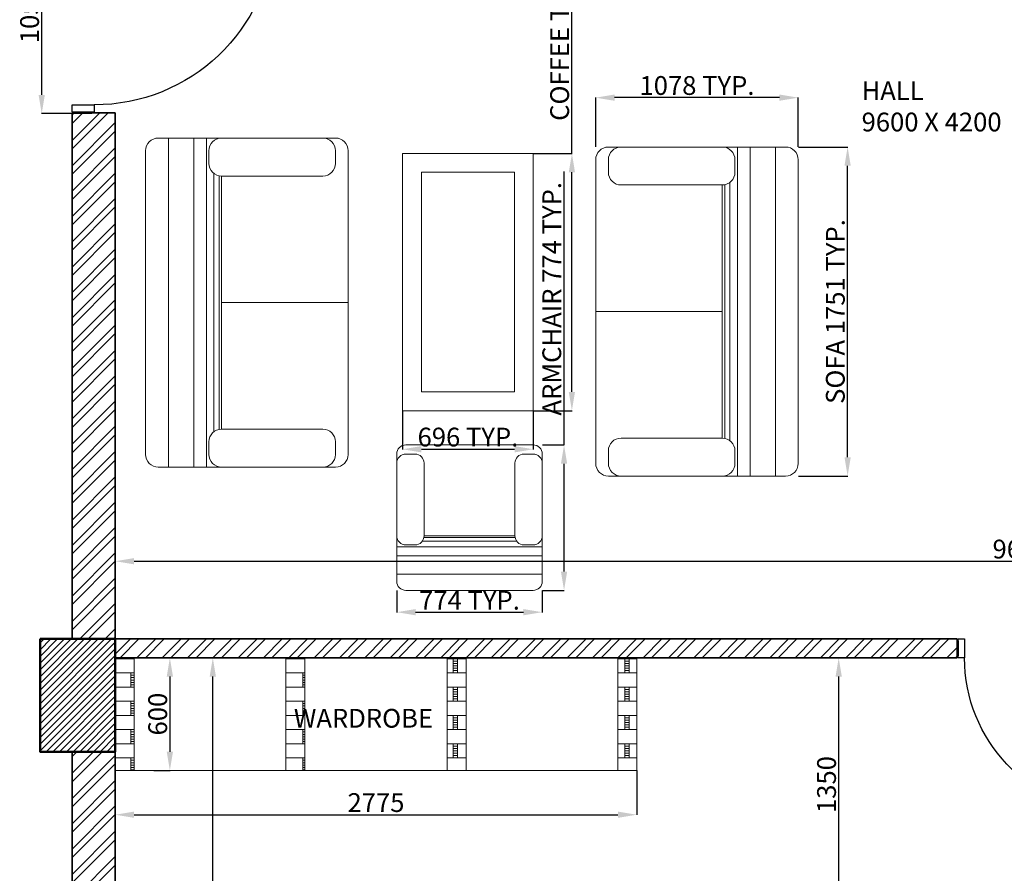
# Model space of a CAD drawing. Units: millimetres. Extents: x -3326 to 29338, y -16792 to 6002.
# Tile 17 of 21: x 17004 to 22244, y -7931 to -3388. Entities that reach past the tile are written whole.
import ezdxf

# ---------------------------------------------------------------- set-up
doc = ezdxf.new("R2010")
doc.units = ezdxf.units.MM
doc.header["$PDMODE"] = 35
doc.header["$PDSIZE"] = 5
for name, color, linetype, lineweight in [('A-ANNO-DIMS', 2, 'Continuous', 13), ('A-AREA-IDEN', 7, 'Continuous', 18), ('A-COLS', 1, 'Continuous', 50), ('A-COLS-PATT', 251, 'Continuous', 13), ('A-DOOR', 3, 'Continuous', 25), ('A-FLOR-CASE', 30, 'Continuous', 18), ('A-FLOR-CASE-PATT', 252, 'Continuous', 13), ('A-WALL', 7, 'Continuous', 35), ('A-WALL-PATT', 252, 'Continuous', 13), ('furn', 28, 'Continuous', 18), ('txt', 7, 'Continuous', 18)]:
    doc.layers.add(name, color=color, linetype=linetype, lineweight=lineweight)
doc.styles.get("Standard").update_dxf_attribs({"font": 'arial.ttf'})
doc.dimstyles.new('ISO-25', dxfattribs={"dimtxt": 100, "dimasz": 100, "dimexe": 1.25, "dimexo": 0.625, "dimtad": 1, "dimtxsty": 'Standard', "dimcen": 2.5, "dimadec": 0, "dimazin": 0, "dimtfac": 1, "dimtmove": 0, "dimatfit": 3, "dimfxl": 1, "dimarcsym": 0})

# ---------------------------------------------------------------- blocks, each defined once
blk = doc.blocks.new('A$C0CE462CD')
for p, q in [((860, 100), (860, 0)), ((860, 0), (893.9, 0))]:
    blk.add_line(p, q)
for points in [[(860, 100), (860, 920), (818.4, 920), (818.4, 100)], [(0, 10), (6.1, 10), (6.1, 90), (0, 90)], [(893.9, 10), (900, 10), (900, 90), (893.9, 90)]]:
    blk.add_lwpolyline(points, close=True)
for points in [[(6.1, 0), (40, 0), (40, 100), (6.1, 100)], [(6.1, 100), (6.1, 0)], [(860, 100), (893.9, 100), (893.9, 0)]]:
    blk.add_lwpolyline(points)
blk.add_arc((859.1, 101.9), 819.1, 92.8508, 180.1309)
blk = doc.blocks.new('sofa-29')
at = {"color": 0, "linetype": 'ByBlock'}
for p, q in [((1.2, 0.8), (0, 0.8)), ((0.6, 0.8), (0.6, 0.3)), ((-0.05, 0.05), (-0.05, 0.75)), ((-0.05, 0.05), (-0.05, 0.75)), ((0, 0.75), (0.05, 0.75)), ((1.2, 0.75), (1.15, 0.75)), ((1.25, 0.05), (1.25, 0.75)), ((0.1, 0.3), (0.1, 0.7)), ((1.1, 0.3), (1.1, 0.7)), ((1.1, 0.29), (0.099, 0.29)), ((1.1, 0.3), (0.1, 0.3)), ((1.25, 0.24), (-0.05, 0.24)), ((0, 0.25), (0.05, 0.25)), ((1.11, 0.27), (0.09, 0.27)), ((1.2, 0.25), (1.15, 0.25)), ((1.25, 0.19), (-0.05, 0.19)), ((1.25, 0.09), (-0.05, 0.09)), ((1.2, 0), (0, 0))]:
    blk.add_line(p, q, dxfattribs=at)
for centre, start, end in [((0, 0.75), 90, 180), ((1.2, 0.75), 0, 90), ((0, 0.7), 90, 180), ((0.05, 0.7), 0, 90), ((1.15, 0.7), 90, 180), ((1.2, 0.7), 0, 90), ((0, 0.3), 180, 270), ((0.05, 0.3), 270, 0), ((1.15, 0.3), 180, 270), ((1.2, 0.3), 270, 0), ((0, 0.05), 180, 270), ((1.2, 0.05), 270, 0)]:
    blk.add_arc(centre, 0.05, start, end, dxfattribs=at)
blk = doc.blocks.new('sofa-30')
at = {"color": 0, "linetype": 'ByBlock'}
for p, q in [((0.7, 0.8), (0, 0.8)), ((-0.05, 0.05), (-0.05, 0.75)), ((-0.05, 0.05), (-0.05, 0.75)), ((0, 0.75), (0.05, 0.75)), ((0.7, 0.75), (0.65, 0.75)), ((0.75, 0.05), (0.75, 0.75)), ((0.1, 0.3), (0.1, 0.7)), ((0.6, 0.3), (0.6, 0.7)), ((0.6, 0.29), (0.099, 0.29)), ((0.6, 0.3), (0.1, 0.3)), ((0.75, 0.24), (-0.05, 0.24)), ((0, 0.25), (0.05, 0.25)), ((0.61, 0.27), (0.09, 0.27)), ((0.7, 0.25), (0.65, 0.25)), ((0.75, 0.19), (-0.05, 0.19)), ((0.75, 0.09), (-0.05, 0.09)), ((0.7, 0), (0, 0))]:
    blk.add_line(p, q, dxfattribs=at)
for centre, start, end in [((0, 0.75), 90, 180), ((0.7, 0.75), 0, 90), ((0, 0.7), 90, 180), ((0.05, 0.7), 0, 90), ((0.65, 0.7), 90, 180), ((0.7, 0.7), 0, 90), ((0, 0.3), 180, 270), ((0.05, 0.3), 270, 0), ((0.65, 0.3), 180, 270), ((0.7, 0.3), 270, 0), ((0, 0.05), 180, 270), ((0.7, 0.05), 270, 0)]:
    blk.add_arc(centre, 0.05, start, end, dxfattribs=at)
blk = doc.blocks.new('*D29')
at = {"layer": 'A-ANNO-DIMS', "color": 0, "lineweight": -2, "transparency": 16777216}
for p, q in [((17512.3, -7384.6), (17512.3, -7620.8)), ((20287.3, -7384.6), (20287.3, -7620.8)), ((17612.3, -7619.5), (20187.3, -7619.5))]:
    blk.add_line(p, q, dxfattribs=at)
at = {"layer": 'A-ANNO-DIMS', "color": 0, "transparency": 16777216}
for points in [[(17612.3, -7602.8), (17612.3, -7636.2), (17512.3, -7619.5)], [(20187.3, -7602.8), (20187.3, -7636.2), (20287.3, -7619.5)]]:
    blk.add_solid(points, dxfattribs=at)
at = {"layer": 'Defpoints', "color": 0, "transparency": 16777216}
for p in [(17512.3, -7384), (20287.3, -7384), (20287.3, -7619.5)]:
    blk.add_point(p, dxfattribs=at)
at = {"layer": 'A-ANNO-DIMS', "color": 0, "transparency": 16777216, "insert": (18899.8, -7567.8), "char_height": 100, "attachment_point": 5}
blk.add_mtext('2775', dxfattribs=at)
blk = doc.blocks.new('*D30')
at = {"layer": 'A-ANNO-DIMS', "color": 0, "lineweight": -2, "transparency": 16777216}
for p, q in [((21362.9, -6784), (21363.6, -6784)), ((21362.3, -8034), (21362.3, -6884)), ((21362.9, -8134), (21363.6, -8134))]:
    blk.add_line(p, q, dxfattribs=at)
at = {"layer": 'A-ANNO-DIMS', "color": 0, "transparency": 16777216}
for points in [[(21345.6, -6884), (21379, -6884), (21362.3, -6784)], [(21345.6, -8034), (21379, -8034), (21362.3, -8134)]]:
    blk.add_solid(points, dxfattribs=at)
at = {"layer": 'Defpoints', "color": 0, "transparency": 16777216}
for p in [(21362.3, -6784), (21362.3, -6784), (21362.3, -8134)]:
    blk.add_point(p, dxfattribs=at)
at = {"layer": 'A-ANNO-DIMS', "color": 0, "transparency": 16777216, "insert": (21310.6, -7459), "char_height": 100, "attachment_point": 5, "rotation": 90}
blk.add_mtext('1350', dxfattribs=at)
blk = doc.blocks.new('*D35')
at = {"layer": 'A-ANNO-DIMS', "color": 0, "lineweight": -2, "transparency": 16777216}
for p, q in [((17512.9, -6784), (18032.6, -6784)), ((18031.3, -10934), (18031.3, -6884)), ((17512.9, -11034), (18032.6, -11034))]:
    blk.add_line(p, q, dxfattribs=at)
at = {"layer": 'A-ANNO-DIMS', "color": 0, "transparency": 16777216}
for points in [[(18014.6, -6884), (18048, -6884), (18031.3, -6784)], [(18014.6, -10934), (18048, -10934), (18031.3, -11034)]]:
    blk.add_solid(points, dxfattribs=at)
at = {"layer": 'Defpoints', "color": 0, "transparency": 16777216}
for p in [(17512.3, -6784), (18031.3, -6784), (17512.3, -11034)]:
    blk.add_point(p, dxfattribs=at)
at = {"layer": 'A-ANNO-DIMS', "color": 0, "transparency": 16777216, "insert": (17979.6, -8909), "char_height": 100, "attachment_point": 5, "rotation": 90}
blk.add_mtext('4250', dxfattribs=at)
blk = doc.blocks.new('*D82')
at = {"layer": 'A-ANNO-DIMS', "color": 0, "lineweight": -2, "transparency": 16777216}
for p, q in [((17718.2, -6784), (17803.9, -6784)), ((17802.7, -6884), (17802.7, -7284)), ((17718.2, -7384), (17803.9, -7384))]:
    blk.add_line(p, q, dxfattribs=at)
at = {"layer": 'A-ANNO-DIMS', "color": 0, "transparency": 16777216}
for points in [[(17786, -6884), (17819.3, -6884), (17802.7, -6784)], [(17786, -7284), (17819.3, -7284), (17802.7, -7384)]]:
    blk.add_solid(points, dxfattribs=at)
at = {"layer": 'Defpoints', "color": 0, "transparency": 16777216}
for p in [(17717.5, -6784), (17717.5, -7384), (17802.7, -7384)]:
    blk.add_point(p, dxfattribs=at)
at = {"layer": 'A-ANNO-DIMS', "color": 0, "transparency": 16777216, "insert": (17751, -7084), "char_height": 100, "attachment_point": 5, "rotation": 90}
blk.add_mtext('600', dxfattribs=at)
blk = doc.blocks.new('*D97')
at = {"layer": 'A-ANNO-DIMS', "color": 0, "lineweight": -2, "transparency": 16777216}
for p, q in [((27152.3, -6119.9), (27152.3, -6271.6)), ((17512.3, -6265.8), (17512.3, -6271.6)), ((17612.3, -6270.4), (27052.3, -6270.4))]:
    blk.add_line(p, q, dxfattribs=at)
at = {"layer": 'A-ANNO-DIMS', "color": 0, "transparency": 16777216}
for points in [[(17612.3, -6253.7), (17612.3, -6287), (17512.3, -6270.4)], [(27052.3, -6253.7), (27052.3, -6287), (27152.3, -6270.4)]]:
    blk.add_solid(points, dxfattribs=at)
at = {"layer": 'Defpoints', "color": 0, "transparency": 16777216}
for p in [(27152.3, -6119.3), (17512.3, -6265.2), (27152.3, -6270.4)]:
    blk.add_point(p, dxfattribs=at)
at = {"layer": 'A-ANNO-DIMS', "color": 0, "transparency": 16777216, "insert": (22332.3, -6218.7), "char_height": 100, "attachment_point": 5}
blk.add_mtext('9640', dxfattribs=at)
blk = doc.blocks.new('TABLE-COFFEE')
for points in [[(0, 1368.6), (695.8, 1368.6), (695.8, 0), (0, 0)], [(100, 1268.6), (595.8, 1268.6), (595.8, 100), (100, 100)]]:
    blk.add_lwpolyline(points, close=True)
blk = doc.blocks.new('*D194')
at = {"layer": 'A-ANNO-DIMS', "color": 0, "lineweight": -2, "transparency": 16777216}
for p, q in [((17281.7, -2835.2), (17119.6, -2835.2)), ((17120.9, -3788.1), (17120.9, -2935.2)), ((17281.7, -3888.1), (17119.6, -3888.1))]:
    blk.add_line(p, q, dxfattribs=at)
at = {"layer": 'A-ANNO-DIMS', "color": 0, "transparency": 16777216}
for points in [[(17104.2, -2935.2), (17137.5, -2935.2), (17120.9, -2835.2)], [(17104.2, -3788.1), (17137.5, -3788.1), (17120.9, -3888.1)]]:
    blk.add_solid(points, dxfattribs=at)
at = {"layer": 'Defpoints', "color": 0, "transparency": 16777216}
for p in [(17120.9, -2835.2), (17282.3, -2835.2), (17282.3, -3888.1)]:
    blk.add_point(p, dxfattribs=at)
at = {"layer": 'A-ANNO-DIMS', "color": 0, "transparency": 16777216, "insert": (17069.1, -3361.6), "char_height": 100, "attachment_point": 5, "rotation": 90}
blk.add_mtext('1053', dxfattribs=at)
blk = doc.blocks.new('*D225')
at = {"layer": 'A-ANNO-DIMS', "color": 0, "lineweight": -2, "transparency": 16777216}
for p, q in [((21147.6, -4065.7), (21410.9, -4065.7)), ((21409.7, -5717.1), (21409.7, -4165.7)), ((21147.6, -5817.1), (21410.9, -5817.1))]:
    blk.add_line(p, q, dxfattribs=at)
at = {"layer": 'A-ANNO-DIMS', "color": 0, "transparency": 16777216}
for points in [[(21393, -4165.7), (21426.3, -4165.7), (21409.7, -4065.7)], [(21393, -5717.1), (21426.3, -5717.1), (21409.7, -5817.1)]]:
    blk.add_solid(points, dxfattribs=at)
at = {"layer": 'Defpoints', "color": 0, "transparency": 16777216}
for p in [(21147, -4065.7), (21409.7, -4065.7), (21147, -5817.1)]:
    blk.add_point(p, dxfattribs=at)
at = {"layer": 'A-ANNO-DIMS', "color": 0, "transparency": 16777216, "insert": (21357.3, -4941.4), "char_height": 100, "attachment_point": 5, "rotation": 90}
blk.add_mtext('SOFA 1751 TYP.', dxfattribs=at)
blk = doc.blocks.new('*D226')
at = {"layer": 'A-ANNO-DIMS', "color": 0, "lineweight": -2, "transparency": 16777216}
for p, q in [((20069.2, -4065.1), (20069.2, -3801.7)), ((21047, -3803), (20169.2, -3803)), ((21147, -4065.1), (21147, -3801.7))]:
    blk.add_line(p, q, dxfattribs=at)
at = {"layer": 'A-ANNO-DIMS', "color": 0, "transparency": 16777216}
for points in [[(20169.2, -3786.3), (20169.2, -3819.6), (20069.2, -3803)], [(21047, -3786.3), (21047, -3819.6), (21147, -3803)]]:
    blk.add_solid(points, dxfattribs=at)
at = {"layer": 'Defpoints', "color": 0, "transparency": 16777216}
for p in [(20069.2, -3803), (20069.2, -4065.7), (21147, -4065.7)]:
    blk.add_point(p, dxfattribs=at)
at = {"layer": 'A-ANNO-DIMS', "color": 0, "transparency": 16777216, "insert": (20608.1, -3751.3), "char_height": 100, "attachment_point": 5}
blk.add_mtext('1078 TYP.', dxfattribs=at)
blk = doc.blocks.new('*D227')
at = {"layer": 'A-ANNO-DIMS', "color": 0, "lineweight": -2, "transparency": 16777216}
for p, q in [((19900.6, -5651.2), (19900.6, -4195.8)), ((19785.1, -5651.2), (19901.9, -5651.2)), ((19900.6, -6325.5), (19900.6, -5751.2)), ((19785.1, -6425.5), (19901.9, -6425.5))]:
    blk.add_line(p, q, dxfattribs=at)
at = {"layer": 'A-ANNO-DIMS', "color": 0, "transparency": 16777216}
for points in [[(19884, -5751.2), (19917.3, -5751.2), (19900.6, -5651.2)], [(19884, -6325.5), (19917.3, -6325.5), (19900.6, -6425.5)]]:
    blk.add_solid(points, dxfattribs=at)
at = {"layer": 'Defpoints', "color": 0, "transparency": 16777216}
for p in [(19784.5, -5651.2), (19900.6, -5651.2), (19784.5, -6425.5)]:
    blk.add_point(p, dxfattribs=at)
at = {"layer": 'A-ANNO-DIMS', "color": 0, "transparency": 16777216, "insert": (19848.3, -4873.5), "char_height": 100, "attachment_point": 5, "rotation": 90}
blk.add_mtext('ARMCHAIR 774 TYP.', dxfattribs=at)
blk = doc.blocks.new('*D228')
at = {"layer": 'A-ANNO-DIMS', "color": 0, "lineweight": -2, "transparency": 16777216}
for p, q in [((19010.3, -6426.1), (19010.3, -6542.8)), ((19784.5, -6426.1), (19784.5, -6542.8)), ((19110.3, -6541.6), (19684.5, -6541.6))]:
    blk.add_line(p, q, dxfattribs=at)
at = {"layer": 'A-ANNO-DIMS', "color": 0, "transparency": 16777216}
for points in [[(19110.3, -6524.9), (19110.3, -6558.2), (19010.3, -6541.6)], [(19684.5, -6524.9), (19684.5, -6558.2), (19784.5, -6541.6)]]:
    blk.add_solid(points, dxfattribs=at)
at = {"layer": 'Defpoints', "color": 0, "transparency": 16777216}
for p in [(19010.3, -6425.5), (19784.5, -6425.5), (19784.5, -6541.6)]:
    blk.add_point(p, dxfattribs=at)
at = {"layer": 'A-ANNO-DIMS', "color": 0, "transparency": 16777216, "insert": (19397.4, -6490.9), "char_height": 100, "attachment_point": 5}
blk.add_mtext('774 TYP.', dxfattribs=at)
blk = doc.blocks.new('*D229')
at = {"layer": 'A-ANNO-DIMS', "color": 0, "lineweight": -2, "transparency": 16777216}
for p, q in [((19942.4, -4100.4), (19942.4, -2271.4)), ((19737.7, -4100.4), (19943.6, -4100.4)), ((19942.4, -5369), (19942.4, -4200.4)), ((19737.7, -5469), (19943.6, -5469))]:
    blk.add_line(p, q, dxfattribs=at)
at = {"layer": 'A-ANNO-DIMS', "color": 0, "transparency": 16777216}
for points in [[(19925.7, -4200.4), (19959, -4200.4), (19942.4, -4100.4)], [(19925.7, -5369), (19959, -5369), (19942.4, -5469)]]:
    blk.add_solid(points, dxfattribs=at)
at = {"layer": 'Defpoints', "color": 0, "transparency": 16777216}
for p in [(19737.1, -4100.4), (19942.4, -4100.4), (19737.1, -5469)]:
    blk.add_point(p, dxfattribs=at)
at = {"layer": 'A-ANNO-DIMS', "color": 0, "transparency": 16777216, "insert": (19890, -3135.9), "char_height": 100, "attachment_point": 5, "rotation": 90}
blk.add_mtext('COFFEE TABLE 1369 TYP.', dxfattribs=at)
blk = doc.blocks.new('*D230')
at = {"layer": 'A-ANNO-DIMS', "color": 0, "lineweight": -2, "transparency": 16777216}
for p, q in [((19041.3, -5469.6), (19041.3, -5675.5)), ((19737.1, -5469.6), (19737.1, -5675.5)), ((19141.3, -5674.3), (19637.1, -5674.3))]:
    blk.add_line(p, q, dxfattribs=at)
at = {"layer": 'A-ANNO-DIMS', "color": 0, "transparency": 16777216}
for points in [[(19141.3, -5657.6), (19141.3, -5691), (19041.3, -5674.3)], [(19637.1, -5657.6), (19637.1, -5691), (19737.1, -5674.3)]]:
    blk.add_solid(points, dxfattribs=at)
at = {"layer": 'Defpoints', "color": 0, "transparency": 16777216}
for p in [(19041.3, -5469), (19737.1, -5469), (19737.1, -5674.3)]:
    blk.add_point(p, dxfattribs=at)
at = {"layer": 'A-ANNO-DIMS', "color": 0, "transparency": 16777216, "insert": (19389.2, -5622.6), "char_height": 100, "attachment_point": 5}
blk.add_mtext('696 TYP.', dxfattribs=at)

msp = doc.modelspace()

# ---------------------------------------------------------------- hatches: boundary and pattern name
at = {"layer": 'A-COLS-PATT'}
h = msp.add_hatch(dxfattribs=at)
h.set_pattern_fill('ANSI31', color=256, scale=8)
h.set_pattern_definition([(45, (-24609, -76.948), (-17.960512, 17.960512), [])])
h.paths.add_polyline_path([(17112.301, -7283.952), (17512.301, -7283.952), (17512.301, -6683.952), (17112.301, -6683.952)])
at = {"layer": 'A-FLOR-CASE-PATT'}
h = msp.add_hatch(dxfattribs=at)
h.set_pattern_fill('BRSTONE', color=256, scale=9)
h.set_pattern_definition([(0, (-10476.645, 1e-12), (0, 75.438), []), (90, (-10270.9, 1e-12), (-114.3, 75.438), [75.438, -75.438]), (90, (-10293.77, 1e-12), (-114.3, 75.438), [75.438, -75.438]), (0, (-10270.905, 12.57), (114.3, 75.438), [-205.74, 22.86]), (0, (-10270.905, 25.146), (114.3, 75.438), [-205.74, 22.86]), (0, (-10270.905, 37.72), (114.3, 75.438), [-205.74, 22.86]), (0, (-10270.905, 50.29), (114.3, 75.438), [-205.74, 22.86]), (0, (-10270.905, 62.865), (114.3, 75.438), [-205.74, 22.86])])
h.paths.add_polyline_path([(17612.301, -6783.952), (17512.301, -6783.952), (17512.301, -7283.952), (17512.301, -7383.952), (17612.301, -7383.952)])
h.paths.add_polyline_path([(18520.634, -6783.952), (18420.634, -6783.952), (18420.634, -7383.952), (18520.634, -7383.952)])
h.paths.add_polyline_path([(19378.967, -6783.952), (19278.967, -6783.952), (19278.967, -7383.952), (19378.967, -7383.952)])
h.paths.add_polyline_path([(20287.301, -6783.952), (20187.301, -6783.952), (20187.301, -7383.952), (20287.301, -7383.952)])
at = {"layer": 'A-WALL-PATT'}
h = msp.add_hatch(dxfattribs=at)
h.set_pattern_fill('ANSI32', color=256, scale=10)
h.set_pattern_definition([(45, (-10476.65, 1e-12), (-67.35192, 67.35192), []), (45, (-10431.74, 1e-12), (-67.35192, 67.35192), [])])
h.paths.add_polyline_path([(29282.301, -7283.952), (28882.301, -7283.952), (28882.301, -7383.952), (29052.301, -7383.952), (29052.301, -10763.952), (29282.301, -10763.952)])
h.paths.add_polyline_path([(29282.301, -11263.952), (29052.301, -11263.952), (29052.301, -12763.952), (29282.301, -12763.952)])
h.paths.add_polyline_path([(25052.301, -11263.952), (25652.301, -11263.952), (25652.301, -11123.904), (25652.289, -11123.904), (25652.289, -11033.952), (25052.301, -11033.952), (24572.301, -11033.952), (24572.301, -11263.952), (24822.301, -11263.952), (24822.301, -12763.952), (25052.301, -12763.952)])
h.paths.add_polyline_path([(26902.301, -11033.952), (26552.301, -11033.952), (26552.301, -11263.952), (26902.301, -11263.952)])
h.paths.add_polyline_path([(21992.301, -6683.952), (21362.301, -6683.952), (17512.301, -6683.952), (17512.301, -6783.952), (21362.301, -6783.952), (21992.301, -6783.952)])
h.paths.add_polyline_path([(17512.301, -7283.952), (17282.301, -7283.952), (17282.301, -12163.952), (17512.301, -12163.952), (17512.301, -11263.952), (18112.301, -11263.952), (18112.301, -11033.952), (17512.301, -11033.952)])
h.paths.add_polyline_path([(21462.301, -8211.864), (21462.064, -8211.864), (21462.064, -8142.609), (21462.301, -8133.952), (21362.301, -8133.952), (21362.301, -8233.952), (21362.301, -11033.952), (21162.301, -11033.952), (21162.301, -11263.952), (21362.301, -11263.952), (21362.301, -12763.952), (21592.301, -12763.952), (21592.301, -11263.952), (21992.301, -11263.952), (21992.301, -11033.952), (21592.301, -11033.952), (21462.301, -11033.952)])
h.paths.add_polyline_path([(24152.301, -8133.952), (23322.301, -8133.952), (23322.301, -7433.952), (23092.301, -7433.952), (23092.301, -8133.952), (22241.021, -8133.952), (22241.021, -8142.609), (22241.182, -8142.609), (22241.182, -8211.864), (22241.021, -8233.952), (23092.301, -8233.952), (23092.301, -10513.206), (23322.301, -10513.206), (23322.301, -8233.952), (24152.301, -8233.952)])
h.paths.add_polyline_path([(25052.301, -8233.952), (25052.301, -8133.952), (24952.301, -8133.952), (24952.301, -11033.952), (25052.301, -11033.952)])
h.paths.add_polyline_path([(23972.301, -11033.952), (23493.251, -11033.952), (23493.251, -11263.952), (23972.301, -11263.952)])
h.paths.add_polyline_path([(23092.301, -11033.952), (22592.301, -11033.952), (22592.301, -11263.952), (23092.301, -11263.952)])
h.paths.add_polyline_path([(28882.301, -11033.952), (28702.301, -11033.952), (28702.301, -11263.952), (28882.301, -11263.952)])
h.paths.add_polyline_path([(17512.301, -3883.952), (17387.589, -3883.952), (17387.589, -3888.07), (17282.301, -3888.07), (17282.301, -6683.952), (17512.301, -6683.952)])
h.paths.add_polyline_path([(21462.301, -2183.952), (21362.301, -2183.952), (21362.301, -2383.952), (17282.301, -2383.952), (17282.301, -2483.952), (17512.301, -2483.952), (21462.301, -2483.952)])
h.paths.add_polyline_path([(17512.301, -2483.952), (17282.301, -2483.952), (17282.301, -2833.952), (17512.301, -2833.952)])
h.paths.add_polyline_path([(21462.301, 1866.048), (21992.301, 1866.048), (21992.301, 2096.048), (21592.301, 2096.048), (21592.301, 3596.048), (21362.301, 3596.048), (21362.301, 1866.048), (21362.301, -1283.952), (21462.301, -1283.952)])
h.paths.add_polyline_path([(17512.301, 1496.048), (17282.301, 1496.048), (17282.301, -1983.952), (17612.301, -1983.952), (17612.301, -1883.952), (17512.301, -1883.952)])
h.paths.add_polyline_path([(17512.301, 3596.048), (17282.301, 3596.048), (17282.301, 2096.048), (17512.301, 2096.048)])
h.paths.add_polyline_path([(18135.023, 2096.048), (17685.023, 2096.048), (17685.023, 1866.048), (18135.023, 1866.048), (18135.023, 1876.048), (18128.942, 1876.048), (18128.942, 1956.048), (18135.023, 1956.048)])
h.paths.add_polyline_path([(19385.023, 2096.048), (19035.023, 2096.048), (19035.023, 1866.048), (19385.023, 1866.048)])
h.paths.add_polyline_path([(21362.301, 2096.048), (21185.023, 2096.048), (21185.023, 1866.048), (21362.301, 1866.048)])
h.paths.add_polyline_path([(23092.301, 2096.048), (22592.301, 2096.048), (22592.301, 1866.048), (23092.301, 1866.048)])
h.paths.add_polyline_path([(23972.301, 2096.048), (23492.301, 2096.048), (23492.301, 1866.048), (23972.301, 1866.048)])
h.paths.add_polyline_path([(23972.301, 2496.048), (23872.301, 2496.048), (23872.301, 2096.048), (23972.301, 2096.048)])
h.paths.add_polyline_path([(22692.301, 2496.048), (22592.301, 2496.048), (22592.301, 2096.048), (22692.301, 2096.048)])
h.paths.add_polyline_path([(23322.301, 1346.048), (23092.301, 1346.048), (23092.301, -1733.952), (23322.301, -1733.952)])
h.paths.add_polyline_path([(23092.301, -933.952), (22262.301, -933.952), (22262.301, -1033.952), (23092.301, -1033.952)])
h.paths.add_polyline_path([(24952.301, -1433.952), (24952.301, -1733.952), (23492.301, -1733.952), (23492.301, -1833.952), (24952.301, -1833.952), (24952.301, -2483.952), (25052.301, -2483.952), (25052.301, -2466.23), (25049.26, -2466.23), (25049.26, -2386.23), (25049.941, -1433.952)])
h.paths.add_polyline_path([(22692.301, -11263.952), (22592.301, -11263.952), (22592.301, -11663.952), (22692.301, -11663.952)])
h.paths.add_polyline_path([(23972.301, -11263.952), (23872.301, -11263.952), (23872.301, -11663.952), (23972.301, -11663.952)])

# ---------------------------------------------------------------- linework, layer by layer
at = {"layer": 'A-COLS'}
msp.add_lwpolyline([(17112.301, -6683.952), (17512.301, -6683.952), (17512.301, -7283.952), (17112.301, -7283.952)], close=True, dxfattribs=at)
at = {"layer": 'A-FLOR-CASE'}
for p, q in [((17612.301, -7383.952), (17612.301, -6783.952)), ((18420.634, -7383.952), (18420.634, -6783.952)), ((18520.634, -7383.952), (18520.634, -6783.952)), ((19278.967, -7383.952), (19278.967, -6783.952)), ((19378.967, -7383.952), (19378.967, -6783.952)), ((20187.301, -7383.952), (20187.301, -6783.952)), ((20287.301, -7383.952), (20287.301, -6783.952)), ((17512.301, -7383.952), (17612.301, -7383.952)), ((17612.301, -7383.952), (20187.301, -7383.952)), ((20187.301, -7383.952), (20287.301, -7383.952))]:
    msp.add_line(p, q, dxfattribs=at)
at = {"layer": 'A-WALL'}
for p, q in [((17282.301, -3883.952), (17282.301, -6683.952)), ((17282.301, -3883.952), (17512.301, -3883.952)), ((17512.301, -3883.952), (17512.301, -11033.952)), ((21362.301, -6683.952), (17512.301, -6683.952)), ((21992.301, -6683.952), (21362.301, -6683.952)), ((21992.301, -6683.952), (21992.301, -6783.952)), ((21362.301, -6783.952), (17512.301, -6783.952)), ((21992.301, -6783.952), (21362.301, -6783.952)), ((17282.301, -7283.952), (17282.301, -12163.952))]:
    msp.add_line(p, q, dxfattribs=at)

# ---------------------------------------------------------------- block references
at = {"layer": 'A-DOOR', "xscale": -1.169867667365197, "yscale": 1.169867667365197, "zscale": 1.169867667365197, "rotation": 270}
msp.add_blockref('A$C0CE462CD', (17282.301, -3888.07), dxfattribs=at)
at = {"layer": 'A-DOOR', "xscale": -1, "rotation": 180}
msp.add_blockref('A$C0CE462CD', (21992.301, -6683.952), dxfattribs=at)
at = {"layer": 'furn', "xscale": 1347.213545272558, "yscale": 1347.213545272558, "zscale": 1347.213545272558}
for p, rotation in [((17673.683, -4085.413), 270), ((21146.962, -5749.701), 89.99999999999999)]:
    msp.add_blockref('sofa-29', p, dxfattribs=dict(at, rotation=rotation))
at = {"layer": 'furn'}
msp.add_blockref('TABLE-COFFEE', (19041.255, -5468.994), dxfattribs=at)
at = {"layer": 'furn', "xscale": 967.7745060020527, "yscale": 967.7745060020527, "zscale": 967.7745060020527}
msp.add_blockref('sofa-30', (19058.658, -6425.45), dxfattribs=at)

# ---------------------------------------------------------------- texts
at = {"layer": 'A-AREA-IDEN', "insert": (21484.165, -3715.873), "char_height": 100, "attachment_point": 1}
msp.add_mtext_dynamic_manual_height_columns('HALL\\P9600 X 4200', width=929.84312, gutter_width=12.5, heights=[0], dxfattribs=at)
at = {"layer": 'txt', "insert": (18462.537, -7056.153), "char_height": 100, "attachment_point": 1}
msp.add_mtext_dynamic_manual_height_columns('WARDROBE', width=1168.90663, gutter_width=12.5, heights=[0], dxfattribs=at)

# ---------------------------------------------------------------- dimensions: what is measured, and where the dimension line sits
at = {"layer": 'A-ANNO-DIMS'}
for base, p1, p2, angle, text, picture, middle in [((19942.36, -4100.372), (19737.067, -5468.994), (19737.067, -4100.372), 90, 'COFFEE TABLE <> TYP.', '*D229', (19889.961, -3135.866)), ((20069.191, -3802.977), (21146.962, -4065.684), (20069.191, -4065.684), 180, '<> TYP.', '*D226', (20608.076, -3751.295)), ((21409.668, -4065.684), (21146.962, -5817.061), (21146.962, -4065.684), 90, 'SOFA <> TYP.', '*D225', (21357.304, -4941.372)), ((19900.622, -5651.231), (19784.489, -6425.45), (19784.489, -5651.231), 90, 'ARMCHAIR <> TYP.', '*D227', (19848.291, -4873.525))]:
    dim = msp.add_linear_dim(base=base, p1=p1, p2=p2, angle=angle, text=text, dimstyle='ISO-25', override={"dimdec": 0, "dimlfac": 1, "dimrnd": 0, "dimzin": 0, "dimdsep": 46, "dimlunit": 2}, dxfattribs=at)
    dim.commit()
    dim.dimension.update_dxf_attribs({"geometry": picture, "text_midpoint": middle})
for base, p1, p2, override, picture, middle in [((17120.859, -2835.189), (17282.301, -3888.07), (17282.301, -2835.189), {"dimdec": 0, "dimlfac": 1, "dimrnd": 0, "dimzin": 0, "dimdsep": 46, "dimlunit": 2}, '*D194', (17069.143, -3361.63)), ((18031.303, -6783.952), (17512.301, -11033.952), (17512.301, -6783.952), {"dimclrd": 0, "dimclre": 0, "dimclrt": 0}, '*D35', (17979.62, -8908.952)), ((17802.657, -7383.952), (17717.542, -6783.952), (17717.542, -7383.952), {"dimclrd": 0, "dimclre": 0, "dimclrt": 0}, '*D82', (17750.974, -7083.952)), ((21362.301, -6783.952), (21362.301, -8133.952), (21362.301, -6783.952), {"dimclrd": 0, "dimclre": 0, "dimclrt": 0}, '*D30', (21310.584, -7458.952))]:
    dim = msp.add_linear_dim(base=base, p1=p1, p2=p2, angle=90, dimstyle='ISO-25', override=override, dxfattribs=at)
    dim.commit()
    dim.dimension.update_dxf_attribs({"geometry": picture, "text_midpoint": middle})
for base, p1, p2, picture, middle in [((19737.067, -5674.287), (19041.255, -5468.994), (19737.067, -5468.994), '*D230', (19389.161, -5622.605)), ((19784.489, -6541.583), (19010.269, -6425.45), (19784.489, -6425.45), '*D228', (19397.379, -6490.924))]:
    dim = msp.add_linear_dim(base=base, p1=p1, p2=p2, text='<> TYP.', dimstyle='ISO-25', override={"dimdec": 0, "dimlfac": 1, "dimrnd": 0, "dimzin": 0, "dimdsep": 46, "dimlunit": 2}, dxfattribs=at)
    dim.commit()
    dim.dimension.update_dxf_attribs({"geometry": picture, "text_midpoint": middle})
for base, p1, p2, picture, middle in [((27152.301, -6270.356), (17512.301, -6265.163), (27152.301, -6119.29), '*D97', (22332.301, -6218.673)), ((20287.301, -7619.511), (17512.301, -7383.952), (20287.301, -7383.952), '*D29', (18899.801, -7567.828))]:
    dim = msp.add_linear_dim(base=base, p1=p1, p2=p2, dimstyle='ISO-25', override={"dimclrd": 0, "dimclre": 0, "dimclrt": 0}, dxfattribs=at)
    dim.commit()
    dim.dimension.update_dxf_attribs({"geometry": picture, "text_midpoint": middle})

doc.saveas('drawing.dxf')
